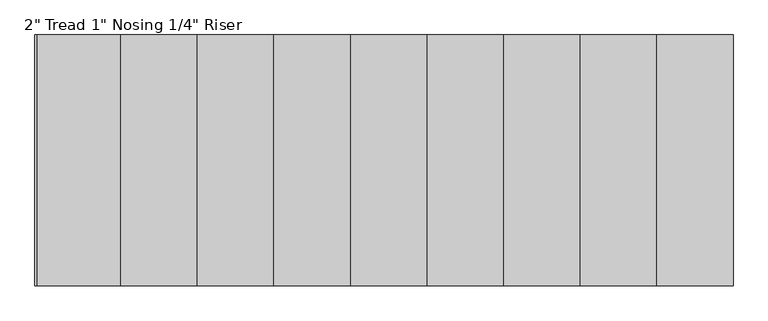
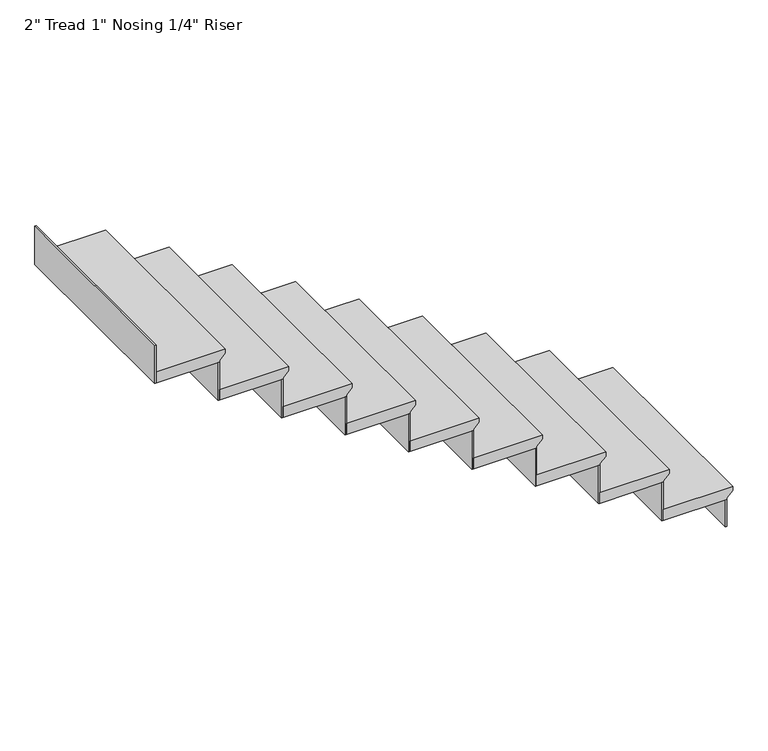
"""IFC4 building model written with IfcOpenShell, lengths in millimetres: stair flight geometry."""

from ifc_helpers import new_model, si_unit, origin, place, context, project, spatial, faceted_brep, source, transform, mapped, element, save


def stair_flight_6f06193a(model_context):
    return source(origin(), model_context, "Body", "Brep", [
        faceted_brep([(-9543.8120641, -2647.9669819, 10369.55), (-9543.8120641, -2647.9669819, 10388.6), (-9543.8120641, -3562.3669819, 10388.6), (-9543.8120641, -3562.3669819, 10369.55), (-9569.2120641, -2647.9669819, 10344.15), (-9569.2120641, -3562.3669819, 10344.15), (-9848.6120641, -2647.9669819, 10388.6), (-9848.6120641, -3562.3669819, 10388.6), (-9569.2120641, -3562.3669819, 10337.8), (-9848.6120641, -3562.3669819, 10337.8), (-9848.6120641, -2647.9669819, 10337.8), (-9569.2120641, -2647.9669819, 10337.8)], [[[0, 1, 2, 3]], [[4, 0, 3, 5]], [[2, 1, 6, 7]], [[8, 9, 10, 11]], [[2, 7, 9, 8, 5, 3]], [[8, 11, 4, 5]], [[6, 1, 0, 4, 11, 10]], [[7, 6, 10, 9]]]),
        faceted_brep([(-9569.2120641, -2647.9669819, 10337.8), (-9569.2120641, -2647.9669819, 10210.8), (-9575.5620641, -2647.9669819, 10210.8), (-9575.5620641, -2647.9669819, 10337.8), (-9569.2120641, -3562.3669819, 10337.8), (-9575.5620641, -3562.3669819, 10337.8), (-9575.5620641, -3562.3669819, 10210.8), (-9569.2120641, -3562.3669819, 10210.8)], [[[0, 1, 2, 3]], [[4, 5, 6, 7]], [[1, 0, 4, 7]], [[2, 1, 7, 6]], [[3, 2, 6, 5]], [[0, 3, 5, 4]]]),
        faceted_brep([(-9848.6120641, -2647.9669819, 10515.6), (-9848.6120641, -2647.9669819, 10337.8), (-9854.9620641, -2647.9669819, 10337.8), (-9854.9620641, -2647.9669819, 10515.6), (-9848.6120641, -3562.3669819, 10515.6), (-9854.9620641, -3562.3669819, 10515.6), (-9854.9620641, -3562.3669819, 10337.8), (-9848.6120641, -3562.3669819, 10337.8)], [[[0, 1, 2, 3]], [[4, 5, 6, 7]], [[1, 0, 4, 7]], [[2, 1, 7, 6]], [[3, 2, 6, 5]], [[0, 3, 5, 4]]]),
        faceted_brep([(-9823.2120641, -3562.3669819, 10566.4), (-9823.2120641, -2647.9669819, 10566.4), (-10128.0120641, -2647.9669819, 10566.4), (-10128.0120641, -3562.3669819, 10566.4), (-9848.6120641, -3562.3669819, 10515.6), (-10128.0120641, -3562.3669819, 10515.6), (-10128.0120641, -2647.9669819, 10515.6), (-9848.6120641, -2647.9669819, 10515.6), (-9848.6120641, -3562.3669819, 10521.95), (-9823.2120641, -3562.3669819, 10547.35), (-9848.6120641, -2647.9669819, 10521.95), (-9823.2120641, -2647.9669819, 10547.35)], [[[0, 1, 2, 3]], [[4, 5, 6, 7]], [[0, 3, 5, 4, 8, 9]], [[4, 7, 10, 8]], [[2, 1, 11, 10, 7, 6]], [[3, 2, 6, 5]], [[11, 1, 0, 9]], [[10, 11, 9, 8]]]),
        faceted_brep([(-10128.0120641, -2647.9669819, 10693.4), (-10128.0120641, -2647.9669819, 10515.6), (-10134.3620641, -2647.9669819, 10515.6), (-10134.3620641, -2647.9669819, 10693.4), (-10128.0120641, -3562.3669819, 10693.4), (-10134.3620641, -3562.3669819, 10693.4), (-10134.3620641, -3562.3669819, 10515.6), (-10128.0120641, -3562.3669819, 10515.6)], [[[0, 1, 2, 3]], [[4, 5, 6, 7]], [[1, 0, 4, 7]], [[2, 1, 7, 6]], [[3, 2, 6, 5]], [[0, 3, 5, 4]]]),
        faceted_brep([(-10102.6120641, -3562.3669819, 10744.2), (-10102.6120641, -2647.9669819, 10744.2), (-10407.4120641, -2647.9669819, 10744.2), (-10407.4120641, -3562.3669819, 10744.2), (-10128.0120641, -3562.3669819, 10693.4), (-10407.4120641, -3562.3669819, 10693.4), (-10407.4120641, -2647.9669819, 10693.4), (-10128.0120641, -2647.9669819, 10693.4), (-10128.0120641, -3562.3669819, 10699.75), (-10102.6120641, -3562.3669819, 10725.15), (-10128.0120641, -2647.9669819, 10699.75), (-10102.6120641, -2647.9669819, 10725.15)], [[[0, 1, 2, 3]], [[4, 5, 6, 7]], [[0, 3, 5, 4, 8, 9]], [[4, 7, 10, 8]], [[2, 1, 11, 10, 7, 6]], [[3, 2, 6, 5]], [[11, 1, 0, 9]], [[10, 11, 9, 8]]]),
        faceted_brep([(-10407.4120641, -2647.9669819, 10871.2), (-10407.4120641, -2647.9669819, 10693.4), (-10413.7620641, -2647.9669819, 10693.4), (-10413.7620641, -2647.9669819, 10871.2), (-10407.4120641, -3562.3669819, 10871.2), (-10413.7620641, -3562.3669819, 10871.2), (-10413.7620641, -3562.3669819, 10693.4), (-10407.4120641, -3562.3669819, 10693.4)], [[[0, 1, 2, 3]], [[4, 5, 6, 7]], [[1, 0, 4, 7]], [[2, 1, 7, 6]], [[3, 2, 6, 5]], [[0, 3, 5, 4]]]),
        faceted_brep([(-10382.0120641, -3562.3669819, 10922.0), (-10382.0120641, -2647.9669819, 10922.0), (-10686.8120641, -2647.9669819, 10922.0), (-10686.8120641, -3562.3669819, 10922.0), (-10407.4120641, -3562.3669819, 10871.2), (-10686.8120641, -3562.3669819, 10871.2), (-10686.8120641, -2647.9669819, 10871.2), (-10407.4120641, -2647.9669819, 10871.2), (-10407.4120641, -3562.3669819, 10877.55), (-10382.0120641, -3562.3669819, 10902.95), (-10407.4120641, -2647.9669819, 10877.55), (-10382.0120641, -2647.9669819, 10902.95)], [[[0, 1, 2, 3]], [[4, 5, 6, 7]], [[0, 3, 5, 4, 8, 9]], [[4, 7, 10, 8]], [[2, 1, 11, 10, 7, 6]], [[3, 2, 6, 5]], [[11, 1, 0, 9]], [[10, 11, 9, 8]]]),
        faceted_brep([(-10686.8120641, -2647.9669819, 11049.0), (-10686.8120641, -2647.9669819, 10871.2), (-10693.1620641, -2647.9669819, 10871.2), (-10693.1620641, -2647.9669819, 11049.0), (-10686.8120641, -3562.3669819, 11049.0), (-10693.1620641, -3562.3669819, 11049.0), (-10693.1620641, -3562.3669819, 10871.2), (-10686.8120641, -3562.3669819, 10871.2)], [[[0, 1, 2, 3]], [[4, 5, 6, 7]], [[1, 0, 4, 7]], [[2, 1, 7, 6]], [[3, 2, 6, 5]], [[0, 3, 5, 4]]]),
        faceted_brep([(-10661.4120641, -3562.3669819, 11099.8), (-10661.4120641, -2647.9669819, 11099.8), (-10966.2120641, -2647.9669819, 11099.8), (-10966.2120641, -3562.3669819, 11099.8), (-10686.8120641, -3562.3669819, 11049.0), (-10966.2120641, -3562.3669819, 11049.0), (-10966.2120641, -2647.9669819, 11049.0), (-10686.8120641, -2647.9669819, 11049.0), (-10686.8120641, -3562.3669819, 11055.35), (-10661.4120641, -3562.3669819, 11080.75), (-10686.8120641, -2647.9669819, 11055.35), (-10661.4120641, -2647.9669819, 11080.75)], [[[0, 1, 2, 3]], [[4, 5, 6, 7]], [[0, 3, 5, 4, 8, 9]], [[4, 7, 10, 8]], [[2, 1, 11, 10, 7, 6]], [[3, 2, 6, 5]], [[11, 1, 0, 9]], [[10, 11, 9, 8]]]),
        faceted_brep([(-10966.2120641, -2647.9669819, 11226.8), (-10966.2120641, -2647.9669819, 11049.0), (-10972.5620641, -2647.9669819, 11049.0), (-10972.5620641, -2647.9669819, 11226.8), (-10966.2120641, -3562.3669819, 11226.8), (-10972.5620641, -3562.3669819, 11226.8), (-10972.5620641, -3562.3669819, 11049.0), (-10966.2120641, -3562.3669819, 11049.0)], [[[0, 1, 2, 3]], [[4, 5, 6, 7]], [[1, 0, 4, 7]], [[2, 1, 7, 6]], [[3, 2, 6, 5]], [[0, 3, 5, 4]]]),
        faceted_brep([(-10940.8120641, -3562.3669819, 11277.6), (-10940.8120641, -2647.9669819, 11277.6), (-11245.6120641, -2647.9669819, 11277.6), (-11245.6120641, -3562.3669819, 11277.6), (-10966.2120641, -3562.3669819, 11226.8), (-11245.6120641, -3562.3669819, 11226.8), (-11245.6120641, -2647.9669819, 11226.8), (-10966.2120641, -2647.9669819, 11226.8), (-10966.2120641, -3562.3669819, 11233.15), (-10940.8120641, -3562.3669819, 11258.55), (-10966.2120641, -2647.9669819, 11233.15), (-10940.8120641, -2647.9669819, 11258.55)], [[[0, 1, 2, 3]], [[4, 5, 6, 7]], [[0, 3, 5, 4, 8, 9]], [[4, 7, 10, 8]], [[2, 1, 11, 10, 7, 6]], [[3, 2, 6, 5]], [[11, 1, 0, 9]], [[10, 11, 9, 8]]]),
        faceted_brep([(-11245.6120641, -2647.9669819, 11404.6), (-11245.6120641, -2647.9669819, 11226.8), (-11251.9620641, -2647.9669819, 11226.8), (-11251.9620641, -2647.9669819, 11404.6), (-11245.6120641, -3562.3669819, 11404.6), (-11251.9620641, -3562.3669819, 11404.6), (-11251.9620641, -3562.3669819, 11226.8), (-11245.6120641, -3562.3669819, 11226.8)], [[[0, 1, 2, 3]], [[4, 5, 6, 7]], [[1, 0, 4, 7]], [[2, 1, 7, 6]], [[3, 2, 6, 5]], [[0, 3, 5, 4]]]),
        faceted_brep([(-11220.2120641, -3562.3669819, 11455.4), (-11220.2120641, -2647.9669819, 11455.4), (-11525.0120641, -2647.9669819, 11455.4), (-11525.0120641, -3562.3669819, 11455.4), (-11245.6120641, -3562.3669819, 11404.6), (-11525.0120641, -3562.3669819, 11404.6), (-11525.0120641, -2647.9669819, 11404.6), (-11245.6120641, -2647.9669819, 11404.6), (-11245.6120641, -3562.3669819, 11410.95), (-11220.2120641, -3562.3669819, 11436.35), (-11245.6120641, -2647.9669819, 11410.95), (-11220.2120641, -2647.9669819, 11436.35)], [[[0, 1, 2, 3]], [[4, 5, 6, 7]], [[0, 3, 5, 4, 8, 9]], [[4, 7, 10, 8]], [[2, 1, 11, 10, 7, 6]], [[3, 2, 6, 5]], [[11, 1, 0, 9]], [[10, 11, 9, 8]]]),
        faceted_brep([(-11525.0120641, -2647.9669819, 11582.4), (-11525.0120641, -2647.9669819, 11404.6), (-11531.3620641, -2647.9669819, 11404.6), (-11531.3620641, -2647.9669819, 11582.4), (-11525.0120641, -3562.3669819, 11582.4), (-11531.3620641, -3562.3669819, 11582.4), (-11531.3620641, -3562.3669819, 11404.6), (-11525.0120641, -3562.3669819, 11404.6)], [[[0, 1, 2, 3]], [[4, 5, 6, 7]], [[1, 0, 4, 7]], [[2, 1, 7, 6]], [[3, 2, 6, 5]], [[0, 3, 5, 4]]]),
        faceted_brep([(-11499.6120641, -3562.3669819, 11633.2), (-11499.6120641, -2647.9669819, 11633.2), (-11804.4120641, -2647.9669819, 11633.2), (-11804.4120641, -3562.3669819, 11633.2), (-11525.0120641, -3562.3669819, 11582.4), (-11804.4120641, -3562.3669819, 11582.4), (-11804.4120641, -2647.9669819, 11582.4), (-11525.0120641, -2647.9669819, 11582.4), (-11525.0120641, -3562.3669819, 11588.75), (-11499.6120641, -3562.3669819, 11614.15), (-11525.0120641, -2647.9669819, 11588.75), (-11499.6120641, -2647.9669819, 11614.15)], [[[0, 1, 2, 3]], [[4, 5, 6, 7]], [[0, 3, 5, 4, 8, 9]], [[4, 7, 10, 8]], [[2, 1, 11, 10, 7, 6]], [[3, 2, 6, 5]], [[11, 1, 0, 9]], [[10, 11, 9, 8]]]),
        faceted_brep([(-12083.8120641, -2647.9669819, 11938.0), (-12083.8120641, -2647.9669819, 11760.2), (-12090.1620641, -2647.9669819, 11760.2), (-12090.1620641, -2647.9669819, 11938.0), (-12083.8120641, -3562.3669819, 11938.0), (-12090.1620641, -3562.3669819, 11938.0), (-12090.1620641, -3562.3669819, 11760.2), (-12083.8120641, -3562.3669819, 11760.2)], [[[0, 1, 2, 3]], [[4, 5, 6, 7]], [[1, 0, 4, 7]], [[2, 1, 7, 6]], [[3, 2, 6, 5]], [[0, 3, 5, 4]]]),
        faceted_brep([(-11804.4120641, -2647.9669819, 11760.2), (-11804.4120641, -2647.9669819, 11582.4), (-11810.7620641, -2647.9669819, 11582.4), (-11810.7620641, -2647.9669819, 11760.2), (-11804.4120641, -3562.3669819, 11760.2), (-11810.7620641, -3562.3669819, 11760.2), (-11810.7620641, -3562.3669819, 11582.4), (-11804.4120641, -3562.3669819, 11582.4)], [[[0, 1, 2, 3]], [[4, 5, 6, 7]], [[1, 0, 4, 7]], [[2, 1, 7, 6]], [[3, 2, 6, 5]], [[0, 3, 5, 4]]]),
        faceted_brep([(-11779.0120641, -3562.3669819, 11811.0), (-11779.0120641, -2647.9669819, 11811.0), (-12058.4120641, -2647.9669819, 11811.0), (-12083.8120641, -2647.9669819, 11811.0), (-12083.8120641, -3562.3669819, 11811.0), (-11804.4120641, -3562.3669819, 11760.2), (-12083.8120641, -3562.3669819, 11760.2), (-12083.8120641, -2647.9669819, 11760.2), (-12058.4120641, -2647.9669819, 11760.2), (-11804.4120641, -2647.9669819, 11760.2), (-11804.4120641, -3562.3669819, 11766.55), (-11779.0120641, -3562.3669819, 11791.95), (-11804.4120641, -2647.9669819, 11766.55), (-11779.0120641, -2647.9669819, 11791.95)], [[[0, 1, 2, 3, 4]], [[5, 6, 7, 8, 9]], [[0, 4, 6, 5, 10, 11]], [[5, 9, 12, 10]], [[2, 1, 13, 12, 9, 8]], [[3, 2, 8, 7]], [[4, 3, 7, 6]], [[13, 1, 0, 11]], [[12, 13, 11, 10]]]),
    ])


if __name__ == "__main__":
    model = new_model("IFC4")
    model_context = context("Model", 3, world=origin())
    ifc_project = project(units=[si_unit("LENGTHUNIT", "METRE", prefix="MILLI")], contexts=[model_context])
    site = spatial("IfcSite", under=ifc_project)
    building = spatial("IfcBuilding", under=site)
    placement = place(None, origin())
    stair_flight_shape = stair_flight_6f06193a(model_context)
    element("IfcStairFlight", 1, ObjectType="2\" Tread 1\" Nosing 1/4\" Riser", at=placement, inside=building, context=model_context, shape_type="MappedRepresentation", body=[
        mapped(stair_flight_shape, transform((0.0, 0.0, 0.0), x_axis=(1.0, 0.0, 0.0), y_axis=(0.0, 1.0, 0.0), z_axis=(0.0, 0.0, 1.0))),
    ])
    save(model, "model.ifc")
